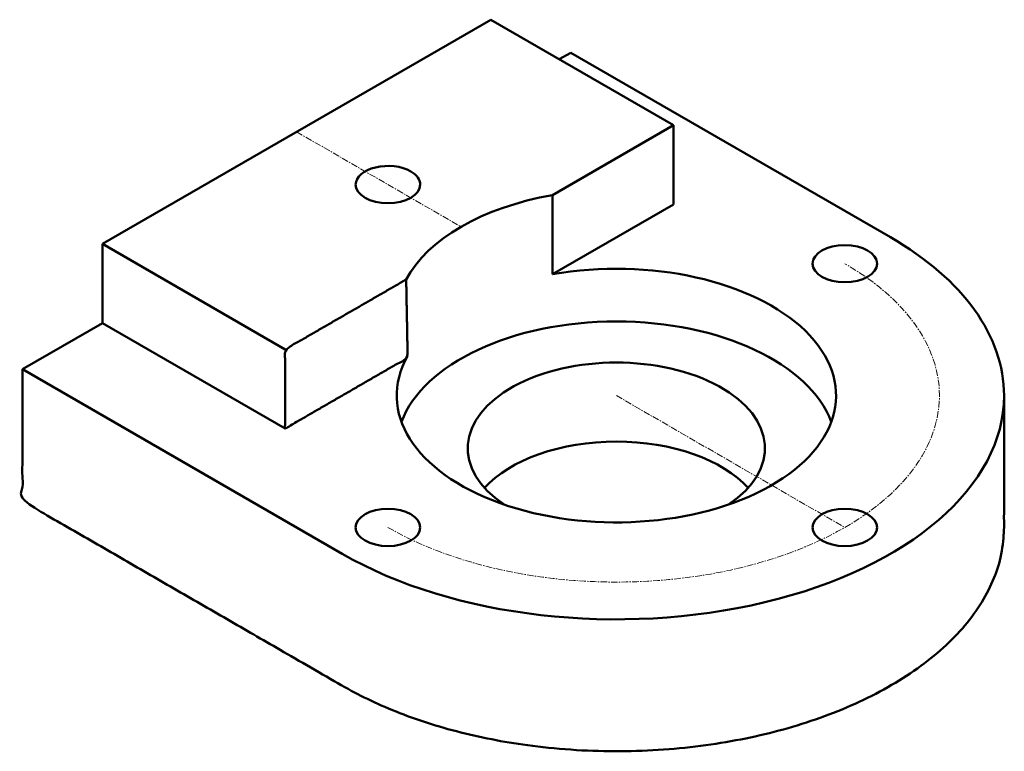
# Model space of a CAD drawing. Units: millimetres. Extents: x 0 to 187, y 15 to 154.
import ezdxf

# ---------------------------------------------------------------- set-up
doc = ezdxf.new("R2010")
doc.units = ezdxf.units.MM
doc.header["$MEASUREMENT"] = 0
doc.linetypes.add('CENTER', pattern=[2, 1.25, -0.25, 0.25, -0.25])
doc.layers.add('M-CNTR', color=4, linetype='CENTER', lineweight=18)
doc.layers.add('M-OUTL', color=7, linetype='Continuous', lineweight=50)

msp = doc.modelspace()

# ---------------------------------------------------------------- linework, layer by layer
at = {"layer": 'M-CNTR'}
for p, q in [((52.44, 132.28), (83.61, 114.28)), ((113.06, 82.28), (156.36, 57.28))]:
    msp.add_line(p, q, dxfattribs=at)
msp.add_ellipse((113.06, 82.28), major_axis=(-61.24, 0), ratio=0.57735, start_param=0.785398, end_param=3.926991, dxfattribs=at)
at = {"layer": 'M-OUTL'}
for p, q in [((15.63, 111.03), (89.24, 153.53)), ((123.88, 133.53), (89.24, 153.53)), ((102.23, 146.03), (104.4, 147.28)), ((165.02, 112.28), (104.4, 147.28)), ((100.93, 120.28), (123.88, 133.53)), ((123.88, 133.53), (123.88, 118.53)), ((100.93, 120.28), (100.93, 105.28)), ((100.93, 105.28), (123.88, 118.53)), ((15.63, 111.03), (50.27, 91.03))]:
    msp.add_line(p, q, dxfattribs=at)
for points in [[(15.63, 111.03), (15.63, 96.03), (50.27, 76.03)], [(15.63, 96.03), (0.47, 87.28), (61.1, 52.28)]]:
    msp.add_lwpolyline(points, dxfattribs=at)
for centre, major_axis, start_param, end_param in [((69.76, 122.28), (6.12, 0), 0.785398, 3.141593), ((69.76, 122.28), (6.12, 0), 0, 0.785398), ((69.76, 122.28), (6.12, 0), 3.141593, 6.283185), ((113.06, 97.28), (-41.64, 0), 5.00783, 5.987744), ((113.06, 82.28), (73.48, 0), 0, 0.785398), ((113.06, 82.28), (-41.64, 0), 5.965931, 11.291015), ((113.06, 72.28), (-41.64, 0), 3.351094, 6.073684), ((113.06, 72.28), (-28.17, 0), 2.425583, 6.999195), ((113.06, 82.28), (73.48, 0), 3.926991, 6.283185), ((113.06, 57.28), (-28.17, 0), 3.620891, 5.803887)]:
    msp.add_ellipse(centre, major_axis=major_axis, ratio=0.57735, start_param=start_param, end_param=end_param, dxfattribs=at)
for centre in [(156.36, 107.28), (69.76, 57.28), (156.36, 57.28)]:
    msp.add_ellipse(centre, major_axis=(-6.12, 0), ratio=0.57735, dxfattribs=at)
for points, weights, knots in [([(73.22, 104.28), (73.36, 97.03), (73.49, 89.78), (73.57, 89.66), (73.64, 89.53), (61.96, 82.78), (50.27, 76.03), (50.27, 83.53), (50.27, 91.03), (61.75, 97.66), (73.22, 104.28)], [1, 1, 1, 0.999984222273, 1, 1, 1, 1, 1, 1, 1], [0, 0, 0, 1, 1, 1.011235, 1.011235, 2.011235, 2.011235, 3.011235, 3.011235, 4.011235, 4.011235, 4.011235]), ([(0.47, 87.28), (0.47, 74.78), (0.47, 62.28), (30.79, 44.78), (61.1, 27.28), (95.82, 7.24), (141.18, 18.09), (186.54, 28.94), (186.54, 57.28), (186.54, 69.78), (186.54, 82.28)], [1, 1, 1, 1, 1, 0.831469612303, 1, 0.831469612303, 1, 1, 1], [0, 0, 0, 1, 1, 2, 2, 3.178097, 3.178097, 4.356194, 4.356194, 5.356194, 5.356194, 5.356194])]:
    msp.add_rational_spline(points, weights, degree=2, knots=knots, dxfattribs=at)

doc.saveas('drawing.dxf')
